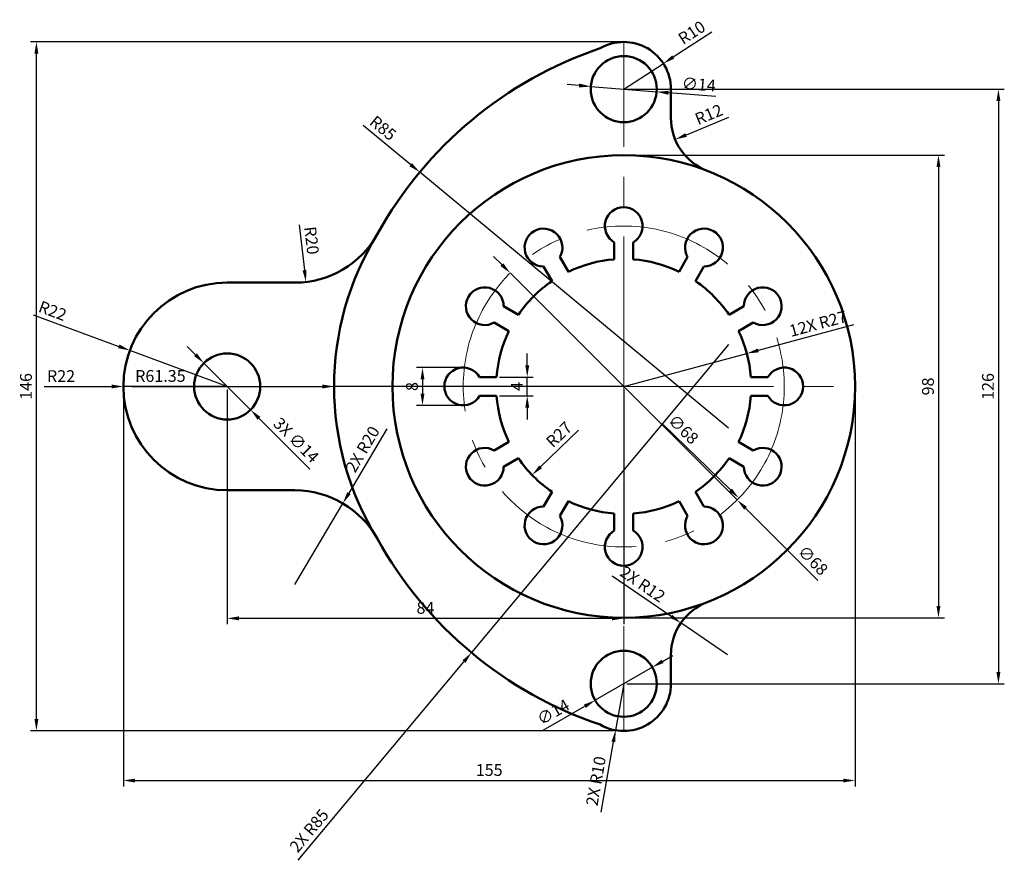
# Model space of a CAD drawing. Units: millimetres. Extents: x -56 to 153, y -43 to 135.
import ezdxf

# ---------------------------------------------------------------- set-up
doc = ezdxf.new("R2010")
doc.units = ezdxf.units.MM
doc.linetypes.add('CENTER', pattern=[50.8, 31.75, -6.35, 6.35, -6.35])
for name, color, linetype, lineweight in [('M-CNTR', 4, 'CENTER', 18), ('M-CONS', 8, 'Continuous', 13), ('M-DIMS', 2, 'Continuous', 25), ('M-OUTL', 7, 'Continuous', 50)]:
    doc.layers.add(name, color=color, linetype=linetype, lineweight=lineweight)
doc.styles.get("Standard").update_dxf_attribs({"font": 'arial.ttf'})
doc.dimstyles.new('ISO-25', dxfattribs={"dimtxt": 2.5, "dimasz": 2.5, "dimexe": 1.25, "dimexo": 0.625, "dimtad": 1, "dimtxsty": 'Standard', "dimcen": 2.5, "dimadec": 0, "dimazin": 0, "dimtfac": 1, "dimtmove": 0, "dimatfit": 3, "dimfxl": 1, "dimarcsym": 0})

# ---------------------------------------------------------------- blocks, each defined once
blk = doc.blocks.new('*U1')
for p, q in [((5.54, 2), (1.93, 2)), ((5.54, -2), (1.93, -2))]:
    blk.add_line(p, q)
blk.add_arc((-1.54, 0), 4, 30, 330)
blk = doc.blocks.new('*U2')
at = {"layer": 'M-OUTL', "color": 0, "linetype": 'ByBlock', "lineweight": -2, "transparency": 16777216}
for p, rotation in [((72.13, 89.86), 269.9999999999998), ((55.9, 85.51), 299.9999999999998), ((88.36, 85.51), 239.9999999999999), ((44.02, 73.63), 329.9999999999999), ((100.25, 73.63), 210), ((104.59, 57.4), 180), ((44.02, 41.16), 30), ((100.25, 41.16), 149.9999999999999), ((55.9, 29.28), 59.99999999999997), ((88.36, 29.28), 119.9999999999999), ((72.13, 24.93), 89.99999999999999)]:
    blk.add_blockref('*U1', p, dxfattribs=dict(at, rotation=rotation))
blk.add_blockref('*U1', (39.67, 57.4), dxfattribs=at)
blk = doc.blocks.new('*D3')
at = {"layer": 'Defpoints', "color": 0, "transparency": 16777216}
for p in [(94.13, 114.29), (83.03, 109.73)]:
    blk.add_point(p, dxfattribs=at)
at = {"layer": 'M-DIMS', "color": 0, "lineweight": -2, "transparency": 16777216}
blk.add_line((94.31, 114.37), (85.34, 110.68), dxfattribs=at)
at = {"layer": 'M-DIMS', "color": 0, "transparency": 16777216}
blk.add_solid([(85.18, 111.07), (85.5, 110.3), (83.03, 109.73)], dxfattribs=at)
at = {"layer": 'M-DIMS', "color": 0, "transparency": 16777216, "insert": (90.27, 114.74), "char_height": 2.5, "attachment_point": 5, "rotation": 22.3178}
blk.add_mtext('R12', dxfattribs=at)
blk = doc.blocks.new('*D4')
at = {"layer": 'Defpoints', "color": 0, "transparency": 16777216}
for p in [(65.15, 120.96), (79.11, 119.83)]:
    blk.add_point(p, dxfattribs=at)
at = {"layer": 'M-DIMS', "color": 0, "lineweight": -2, "transparency": 16777216}
for p, q in [((62.66, 121.16), (60.17, 121.37)), ((65.15, 120.96), (79.11, 119.83)), ((91.61, 118.81), (81.6, 119.63))]:
    blk.add_line(p, q, dxfattribs=at)
blk.add_arc((72.13, 120.4), 7, 345.1248, 354.8843, dxfattribs=at)
at = {"layer": 'M-DIMS', "color": 0, "transparency": 16777216}
for points in [[(62.7, 121.58), (62.63, 120.75), (65.15, 120.96)], [(81.63, 120.04), (81.57, 119.21), (79.11, 119.83)]]:
    blk.add_solid(points, dxfattribs=at)
at = {"layer": 'M-DIMS', "color": 0, "transparency": 16777216, "insert": (88.01, 121.08), "char_height": 2.5, "attachment_point": 5, "rotation": 355.3562}
blk.add_mtext('∅14', dxfattribs=at)
blk = doc.blocks.new('*D5')
at = {"layer": 'Defpoints', "color": 0, "transparency": 16777216}
for p in [(80.52, 125.84), (72.13, 120.4)]:
    blk.add_point(p, dxfattribs=at)
at = {"layer": 'M-DIMS', "color": 0, "lineweight": -2, "transparency": 16777216}
for p, q in [((90.77, 132.49), (82.62, 127.2)), ((72.13, 120.4), (80.52, 125.84))]:
    blk.add_line(p, q, dxfattribs=at)
at = {"layer": 'M-DIMS', "color": 0, "transparency": 16777216}
blk.add_solid([(82.39, 127.55), (82.84, 126.85), (80.52, 125.84)], dxfattribs=at)
at = {"layer": 'M-DIMS', "color": 0, "transparency": 16777216, "insert": (86.71, 132.12), "char_height": 2.5, "attachment_point": 5, "rotation": 32.9791}
blk.add_mtext('R10', dxfattribs=at)
blk = doc.blocks.new('*D6')
at = {"layer": 'Defpoints', "color": 0, "transparency": 16777216}
for p in [(72.13, 120.4), (72.13, -5.6), (151.5, -5.6)]:
    blk.add_point(p, dxfattribs=at)
at = {"layer": 'M-DIMS', "color": 0, "lineweight": -2, "transparency": 16777216}
for p, q in [((72.76, 120.4), (152.75, 120.4)), ((151.5, 117.9), (151.5, -3.1)), ((72.76, -5.6), (152.75, -5.6))]:
    blk.add_line(p, q, dxfattribs=at)
at = {"layer": 'M-DIMS', "color": 0, "transparency": 16777216}
for points in [[(151.08, 117.9), (151.92, 117.9), (151.5, 120.4)], [(151.08, -3.1), (151.92, -3.1), (151.5, -5.6)]]:
    blk.add_solid(points, dxfattribs=at)
at = {"layer": 'M-DIMS', "color": 0, "transparency": 16777216, "insert": (149.6, 57.4), "char_height": 2.5, "attachment_point": 5, "rotation": 90}
blk.add_mtext('126', dxfattribs=at)
blk = doc.blocks.new('*D7')
at = {"layer": 'Defpoints', "color": 0, "transparency": 16777216}
for p in [(72.13, 106.4), (72.13, 8.4), (138.8, 8.4)]:
    blk.add_point(p, dxfattribs=at)
at = {"layer": 'M-DIMS', "color": 0, "lineweight": -2, "transparency": 16777216}
for p, q in [((72.76, 106.4), (140.05, 106.4)), ((138.8, 103.9), (138.8, 10.9)), ((72.76, 8.4), (140.05, 8.4))]:
    blk.add_line(p, q, dxfattribs=at)
at = {"layer": 'M-DIMS', "color": 0, "transparency": 16777216}
for points in [[(138.38, 103.9), (139.22, 103.9), (138.8, 106.4)], [(138.38, 10.9), (139.22, 10.9), (138.8, 8.4)]]:
    blk.add_solid(points, dxfattribs=at)
at = {"layer": 'M-DIMS', "color": 0, "transparency": 16777216, "insert": (136.9, 57.4), "char_height": 2.5, "attachment_point": 5, "rotation": 90}
blk.add_mtext('98', dxfattribs=at)
blk = doc.blocks.new('*D8')
at = {"layer": 'Defpoints', "color": 0, "transparency": 16777216}
for p in [(72.13, 57.4), (52.72, 38.63)]:
    blk.add_point(p, dxfattribs=at)
at = {"layer": 'M-DIMS', "color": 0, "lineweight": -2, "transparency": 16777216}
blk.add_line((62.56, 48.14), (54.52, 40.37), dxfattribs=at)
at = {"layer": 'M-DIMS', "color": 0, "transparency": 16777216}
blk.add_solid([(54.23, 40.66), (54.81, 40.07), (52.72, 38.63)], dxfattribs=at)
at = {"layer": 'M-DIMS', "color": 0, "transparency": 16777216, "insert": (58.65, 46.98), "char_height": 2.5, "attachment_point": 5, "rotation": 44.0365}
blk.add_mtext('R27', dxfattribs=at)
blk = doc.blocks.new('*D9')
at = {"layer": 'Defpoints', "color": 0, "transparency": 16777216}
for p in [(47.72, 81.07), (96.54, 33.73)]:
    blk.add_point(p, dxfattribs=at)
at = {"layer": 'M-DIMS', "color": 0, "lineweight": -2, "transparency": 16777216}
blk.add_line((80.47, 49.31), (94.74, 35.47), dxfattribs=at)
at = {"layer": 'M-DIMS', "color": 0, "transparency": 16777216}
blk.add_solid([(95.03, 35.76), (94.45, 35.17), (96.54, 33.73)], dxfattribs=at)
at = {"layer": 'M-DIMS', "color": 0, "transparency": 16777216, "insert": (84.55, 48.09), "char_height": 2.5, "attachment_point": 5, "rotation": 315.8786}
blk.add_mtext('∅68', dxfattribs=at)
blk = doc.blocks.new('*D10')
at = {"layer": 'Defpoints', "color": 0, "transparency": 16777216}
for p in [(-32.5, 65.03), (-11.87, 57.4)]:
    blk.add_point(p, dxfattribs=at)
at = {"layer": 'M-DIMS', "color": 0, "lineweight": -2, "transparency": 16777216}
for p, q in [((-52.98, 72.6), (-34.85, 65.89)), ((-11.87, 57.4), (-32.5, 65.03))]:
    blk.add_line(p, q, dxfattribs=at)
at = {"layer": 'M-DIMS', "color": 0, "transparency": 16777216}
blk.add_solid([(-34.7, 66.29), (-34.99, 65.5), (-32.5, 65.03)], dxfattribs=at)
at = {"layer": 'M-DIMS', "color": 0, "transparency": 16777216, "insert": (-48.96, 73.12), "char_height": 2.5, "attachment_point": 5, "rotation": 339.7013}
blk.add_mtext('R22', dxfattribs=at)
blk = doc.blocks.new('*D11')
at = {"layer": 'Defpoints', "color": 0, "transparency": 16777216}
for p in [(2.49, 99.4), (4.81, 79.53)]:
    blk.add_point(p, dxfattribs=at)
at = {"layer": 'M-DIMS', "color": 0, "lineweight": -2, "transparency": 16777216}
blk.add_line((3.39, 91.66), (4.52, 82.01), dxfattribs=at)
at = {"layer": 'M-DIMS', "color": 0, "transparency": 16777216}
blk.add_solid([(4.93, 82.06), (4.1, 81.97), (4.81, 79.53)], dxfattribs=at)
at = {"layer": 'M-DIMS', "color": 0, "transparency": 16777216, "insert": (5.7, 88.3), "char_height": 2.5, "attachment_point": 5, "rotation": 276.6683}
blk.add_mtext('R20', dxfattribs=at)
blk = doc.blocks.new('*D12')
at = {"layer": 'Defpoints', "color": 0, "transparency": 16777216}
for p in [(-11.87, 57.4), (72.13, 57.4), (-11.87, 8.26)]:
    blk.add_point(p, dxfattribs=at)
at = {"layer": 'M-DIMS', "color": 0, "lineweight": -2, "transparency": 16777216}
for p, q in [((-11.87, 56.77), (-11.87, 7.01)), ((72.13, 56.77), (72.13, 7.01)), ((69.63, 8.26), (-9.37, 8.26))]:
    blk.add_line(p, q, dxfattribs=at)
at = {"layer": 'M-DIMS', "color": 0, "transparency": 16777216}
for points in [[(-9.37, 8.68), (-9.37, 7.84), (-11.87, 8.26)], [(69.63, 8.68), (69.63, 7.84), (72.13, 8.26)]]:
    blk.add_solid(points, dxfattribs=at)
at = {"layer": 'M-DIMS', "color": 0, "transparency": 16777216, "insert": (30.13, 10.16), "char_height": 2.5, "attachment_point": 5}
blk.add_mtext('84', dxfattribs=at)
blk = doc.blocks.new('*D13')
at = {"layer": 'Defpoints', "color": 0, "transparency": 16777216}
for p in [(38.37, 61.39), (29.5, 53.39), (38.37, 53.39)]:
    blk.add_point(p, dxfattribs=at)
at = {"layer": 'M-DIMS', "color": 0, "lineweight": -2, "transparency": 16777216}
for p, q in [((37.74, 61.39), (28.25, 61.39)), ((29.5, 58.89), (29.5, 55.89)), ((37.74, 53.39), (28.25, 53.39))]:
    blk.add_line(p, q, dxfattribs=at)
at = {"layer": 'M-DIMS', "color": 0, "transparency": 16777216}
for points in [[(29.09, 58.89), (29.92, 58.89), (29.5, 61.39)], [(29.09, 55.89), (29.92, 55.89), (29.5, 53.39)]]:
    blk.add_solid(points, dxfattribs=at)
at = {"layer": 'M-DIMS', "color": 0, "transparency": 16777216, "insert": (27.6, 57.39), "char_height": 2.5, "attachment_point": 5, "rotation": 90}
blk.add_mtext('8', dxfattribs=at)
blk = doc.blocks.new('*D14')
at = {"layer": 'Defpoints', "color": 0, "transparency": 16777216}
for p in [(45.21, 59.4), (51.69, 59.4), (45.21, 55.4)]:
    blk.add_point(p, dxfattribs=at)
at = {"layer": 'M-DIMS', "color": 0, "lineweight": -2, "transparency": 16777216}
for p, q in [((51.69, 61.9), (51.69, 64.4)), ((45.83, 59.4), (52.94, 59.4)), ((51.69, 55.4), (51.69, 59.4)), ((45.83, 55.4), (52.94, 55.4)), ((51.69, 52.9), (51.69, 50.4))]:
    blk.add_line(p, q, dxfattribs=at)
at = {"layer": 'M-DIMS', "color": 0, "transparency": 16777216}
for points in [[(51.28, 61.9), (52.11, 61.9), (51.69, 59.4)], [(51.28, 52.9), (52.11, 52.9), (51.69, 55.4)]]:
    blk.add_solid(points, dxfattribs=at)
at = {"layer": 'M-DIMS', "color": 0, "transparency": 16777216, "insert": (49.82, 57.4), "char_height": 2.5, "attachment_point": 5, "rotation": 90}
blk.add_mtext('4', dxfattribs=at)
blk = doc.blocks.new('*D15')
at = {"layer": 'Defpoints', "color": 0, "transparency": 16777216}
for p in [(28.92, 102.8), (94.34, 48.53)]:
    blk.add_point(p, dxfattribs=at)
at = {"layer": 'M-DIMS', "color": 0, "lineweight": -2, "transparency": 16777216}
for p, q in [((16.94, 112.75), (27, 104.4)), ((94.34, 48.53), (28.92, 102.8))]:
    blk.add_line(p, q, dxfattribs=at)
at = {"layer": 'M-DIMS', "color": 0, "transparency": 16777216}
blk.add_solid([(27.27, 104.72), (26.73, 104.08), (28.92, 102.8)], dxfattribs=at)
at = {"layer": 'M-DIMS', "color": 0, "transparency": 16777216, "insert": (20.94, 111.9), "char_height": 2.5, "attachment_point": 5, "rotation": 320.3196}
blk.add_mtext('R85', dxfattribs=at)
blk = doc.blocks.new('*D16')
at = {"layer": 'Defpoints', "color": 0, "transparency": 16777216}
for p in [(78.19, -2.1), (66.07, -9.11)]:
    blk.add_point(p, dxfattribs=at)
at = {"layer": 'M-DIMS', "color": 0, "lineweight": -2, "transparency": 16777216}
for p, q in [((80.36, -0.85), (82.52, 0.4)), ((78.19, -2.1), (66.07, -9.11)), ((55.07, -15.46), (63.91, -10.36))]:
    blk.add_line(p, q, dxfattribs=at)
at = {"layer": 'M-DIMS', "color": 0, "transparency": 16777216}
for points in [[(80.15, -0.49), (80.57, -1.21), (78.19, -2.1)], [(63.7, -10), (64.11, -10.72), (66.07, -9.11)]]:
    blk.add_solid(points, dxfattribs=at)
at = {"layer": 'M-DIMS', "color": 0, "transparency": 16777216, "insert": (57.35, -11.87), "char_height": 2.5, "attachment_point": 5, "rotation": 30.014}
blk.add_mtext('∅14', dxfattribs=at)
blk = doc.blocks.new('MOUNT-HOLE-D14')
blk.add_circle((7, 7), 7)
blk = doc.blocks.new('*D18')
at = {"layer": 'Defpoints', "color": 0, "transparency": 16777216}
for p in [(-52.28, 130.4), (72.13, 130.4), (72.13, -15.6)]:
    blk.add_point(p, dxfattribs=at)
at = {"layer": 'M-DIMS', "color": 0, "lineweight": -2, "transparency": 16777216}
for p, q in [((71.51, 130.4), (-53.53, 130.4)), ((-52.28, -13.1), (-52.28, 127.9)), ((71.51, -15.6), (-53.53, -15.6))]:
    blk.add_line(p, q, dxfattribs=at)
at = {"layer": 'M-DIMS', "color": 0, "transparency": 16777216}
for points in [[(-52.7, 127.9), (-51.87, 127.9), (-52.28, 130.4)], [(-52.7, -13.1), (-51.87, -13.1), (-52.28, -15.6)]]:
    blk.add_solid(points, dxfattribs=at)
at = {"layer": 'M-DIMS', "color": 0, "transparency": 16777216, "insert": (-54.18, 57.4), "char_height": 2.5, "attachment_point": 5, "rotation": 90}
blk.add_mtext('146', dxfattribs=at)
blk = doc.blocks.new('*D19')
at = {"layer": 'Defpoints', "color": 0, "transparency": 16777216}
for p in [(-33.87, 57.4), (121.13, 57.4), (121.13, -26.1)]:
    blk.add_point(p, dxfattribs=at)
at = {"layer": 'M-DIMS', "color": 0, "lineweight": -2, "transparency": 16777216}
for p, q in [((-33.87, 56.77), (-33.87, -27.35)), ((121.13, 56.77), (121.13, -27.35)), ((-31.37, -26.1), (118.63, -26.1))]:
    blk.add_line(p, q, dxfattribs=at)
at = {"layer": 'M-DIMS', "color": 0, "transparency": 16777216}
for points in [[(-31.37, -25.69), (-31.37, -26.52), (-33.87, -26.1)], [(118.63, -25.69), (118.63, -26.52), (121.13, -26.1)]]:
    blk.add_solid(points, dxfattribs=at)
at = {"layer": 'M-DIMS', "color": 0, "transparency": 16777216, "insert": (43.63, -24.2), "char_height": 2.5, "attachment_point": 5}
blk.add_mtext('155', dxfattribs=at)
blk = doc.blocks.new('*D20')
at = {"layer": 'Defpoints', "color": 0, "transparency": 16777216}
for p in [(94.34, 66.26), (39.88, 1)]:
    blk.add_point(p, dxfattribs=at)
at = {"layer": 'M-DIMS', "color": 0, "lineweight": -2, "transparency": 16777216}
for p, q in [((94.34, 66.26), (39.88, 1)), ((3.15, -43.01), (38.28, -0.92))]:
    blk.add_line(p, q, dxfattribs=at)
at = {"layer": 'M-DIMS', "color": 0, "transparency": 16777216}
blk.add_solid([(37.96, -0.65), (38.6, -1.18), (39.88, 1)], dxfattribs=at)
at = {"layer": 'M-DIMS', "color": 0, "transparency": 16777216, "insert": (5.74, -36.93), "char_height": 2.5, "attachment_point": 5, "rotation": 50.1525}
blk.add_mtext('2X R85', dxfattribs=at)
blk = doc.blocks.new('*D21')
at = {"layer": 'Defpoints', "color": 0, "transparency": 16777216}
for p in [(10.78, 57.39), (72.13, 57.4)]:
    blk.add_point(p, dxfattribs=at)
at = {"layer": 'M-DIMS', "color": 0, "lineweight": -2, "transparency": 16777216}
for p, q in [((-32.07, 57.39), (8.28, 57.39)), ((72.13, 57.4), (10.78, 57.39))]:
    blk.add_line(p, q, dxfattribs=at)
at = {"layer": 'M-DIMS', "color": 0, "transparency": 16777216}
blk.add_solid([(8.28, 57.81), (8.28, 56.98), (10.78, 57.39)], dxfattribs=at)
at = {"layer": 'M-DIMS', "color": 0, "transparency": 16777216, "insert": (-26.02, 59.3), "char_height": 2.5, "attachment_point": 5, "rotation": 0.0003}
blk.add_mtext('R61.35', dxfattribs=at)
blk = doc.blocks.new('*D22')
at = {"layer": 'Defpoints', "color": 0, "transparency": 16777216}
for p in [(48.09, 81.44), (96.17, 33.35)]:
    blk.add_point(p, dxfattribs=at)
at = {"layer": 'M-DIMS', "color": 0, "lineweight": -2, "transparency": 16777216}
for p, q in [((46.32, 83.21), (44.55, 84.97)), ((48.09, 81.44), (96.17, 33.35)), ((113.27, 16.26), (97.94, 31.59))]:
    blk.add_line(p, q, dxfattribs=at)
at = {"layer": 'M-DIMS', "color": 0, "transparency": 16777216}
for points in [[(46.62, 83.5), (46.03, 82.91), (48.09, 81.44)], [(98.24, 31.88), (97.65, 31.29), (96.17, 33.35)]]:
    blk.add_solid(points, dxfattribs=at)
at = {"layer": 'M-DIMS', "color": 0, "transparency": 16777216, "insert": (111.99, 20.32), "char_height": 2.5, "attachment_point": 5, "rotation": 314.9991}
blk.add_mtext('∅68', dxfattribs=at)
blk = doc.blocks.new('*D23')
at = {"layer": 'Defpoints', "color": 0, "transparency": 16777216}
for p in [(98.21, 64.38), (72.13, 57.4)]:
    blk.add_point(p, dxfattribs=at)
at = {"layer": 'M-DIMS', "color": 0, "lineweight": -2, "transparency": 16777216}
for p, q in [((120.77, 70.43), (100.63, 65.03)), ((72.13, 57.4), (98.21, 64.38))]:
    blk.add_line(p, q, dxfattribs=at)
at = {"layer": 'M-DIMS', "color": 0, "transparency": 16777216}
blk.add_solid([(100.52, 65.43), (100.73, 64.63), (98.21, 64.38)], dxfattribs=at)
at = {"layer": 'M-DIMS', "color": 0, "transparency": 16777216, "insert": (113.37, 70.39), "char_height": 2.5, "attachment_point": 5, "rotation": 14.9992}
blk.add_mtext('12X R27', dxfattribs=at)
blk = doc.blocks.new('*D24')
at = {"layer": 'Defpoints', "color": 0, "transparency": 16777216}
for p in [(-33.87, 57.39), (-11.87, 57.4)]:
    blk.add_point(p, dxfattribs=at)
at = {"layer": 'M-DIMS', "color": 0, "lineweight": -2, "transparency": 16777216}
for p, q in [((-50.67, 57.39), (-36.37, 57.39)), ((-11.87, 57.4), (-33.87, 57.39))]:
    blk.add_line(p, q, dxfattribs=at)
at = {"layer": 'M-DIMS', "color": 0, "transparency": 16777216}
blk.add_solid([(-36.37, 57.81), (-36.37, 56.98), (-33.87, 57.39)], dxfattribs=at)
at = {"layer": 'M-DIMS', "color": 0, "transparency": 16777216, "insert": (-47.07, 59.27), "char_height": 2.5, "attachment_point": 5, "rotation": 0.001}
blk.add_mtext('R22', dxfattribs=at)
blk = doc.blocks.new('*D25')
at = {"layer": 'Defpoints', "color": 0, "transparency": 16777216}
for p in [(12.64, 32.63), (2.49, 15.4)]:
    blk.add_point(p, dxfattribs=at)
at = {"layer": 'M-DIMS', "color": 0, "lineweight": -2, "transparency": 16777216}
for p, q in [((21.94, 48.4), (13.91, 34.78)), ((2.49, 15.4), (12.64, 32.63))]:
    blk.add_line(p, q, dxfattribs=at)
at = {"layer": 'M-DIMS', "color": 0, "transparency": 16777216}
blk.add_solid([(13.55, 34.99), (14.27, 34.57), (12.64, 32.63)], dxfattribs=at)
at = {"layer": 'M-DIMS', "color": 0, "transparency": 16777216, "insert": (17.09, 43.93), "char_height": 2.5, "attachment_point": 5, "rotation": 59.4893}
blk.add_mtext('2X R20', dxfattribs=at)
blk = doc.blocks.new('*D26')
at = {"layer": 'Defpoints', "color": 0, "transparency": 16777216}
for p in [(84.23, 7.29), (94.13, 0.5)]:
    blk.add_point(p, dxfattribs=at)
at = {"layer": 'M-DIMS', "color": 0, "lineweight": -2, "transparency": 16777216}
for p, q in [((69.71, 17.24), (82.17, 8.7)), ((94.13, 0.5), (84.23, 7.29))]:
    blk.add_line(p, q, dxfattribs=at)
at = {"layer": 'M-DIMS', "color": 0, "transparency": 16777216}
blk.add_solid([(82.41, 9.04), (81.94, 8.36), (84.23, 7.29)], dxfattribs=at)
at = {"layer": 'M-DIMS', "color": 0, "transparency": 16777216, "insert": (75.97, 15.23), "char_height": 2.5, "attachment_point": 5, "rotation": 325.5709}
blk.add_mtext('2X R12', dxfattribs=at)
blk = doc.blocks.new('*D27')
at = {"layer": 'Defpoints', "color": 0, "transparency": 16777216}
for p in [(72.13, -5.6), (70.4, -15.45)]:
    blk.add_point(p, dxfattribs=at)
at = {"layer": 'M-DIMS', "color": 0, "lineweight": -2, "transparency": 16777216}
for p, q in [((72.13, -5.6), (70.4, -15.45)), ((67.33, -32.81), (69.96, -17.91))]:
    blk.add_line(p, q, dxfattribs=at)
at = {"layer": 'M-DIMS', "color": 0, "transparency": 16777216}
blk.add_solid([(69.55, -17.84), (70.37, -17.99), (70.4, -15.45)], dxfattribs=at)
at = {"layer": 'M-DIMS', "color": 0, "transparency": 16777216, "insert": (66.56, -26.27), "char_height": 2.5, "attachment_point": 5, "rotation": 80.0009}
blk.add_mtext('2X R10', dxfattribs=at)
blk = doc.blocks.new('*D28')
at = {"layer": 'Defpoints', "color": 0, "transparency": 16777216}
for p in [(-16.82, 62.35), (-6.92, 52.45)]:
    blk.add_point(p, dxfattribs=at)
at = {"layer": 'M-DIMS', "color": 0, "lineweight": -2, "transparency": 16777216}
for p, q in [((-18.59, 64.11), (-20.35, 65.88)), ((-16.82, 62.35), (-6.92, 52.45)), ((5.65, 39.87), (-5.15, 50.68))]:
    blk.add_line(p, q, dxfattribs=at)
at = {"layer": 'M-DIMS', "color": 0, "transparency": 16777216}
for points in [[(-18.29, 64.41), (-18.88, 63.82), (-16.82, 62.35)], [(-4.86, 50.97), (-5.45, 50.38), (-6.92, 52.45)]]:
    blk.add_solid(points, dxfattribs=at)
at = {"layer": 'M-DIMS', "color": 0, "transparency": 16777216, "insert": (2.53, 45.79), "char_height": 2.5, "attachment_point": 5, "rotation": 314.9956}
blk.add_mtext('3X ∅14', dxfattribs=at)

msp = doc.modelspace()

# ---------------------------------------------------------------- linework, layer by layer
at = {"layer": 'M-CNTR'}
for p, q in [((72.131, 120.395), (72.131, 130.395)), ((72.131, 57.395), (72.131, 120.395)), ((10.784, 57.395), (-41.783, 57.395)), ((72.131, 57.395), (10.784, 57.395)), ((72.131, 57.395), (72.131, -5.605)), ((72.131, 57.395), (121.131, 57.395)), ((72.131, -5.605), (72.131, -15.605))]:
    msp.add_line(p, q, dxfattribs=at)
msp.add_circle((72.131, 57.395), 34, dxfattribs=at)
at = {"layer": 'M-CONS'}
for p, q in [((72.131, 120.395), (72.131, 120.395)), ((72.131, 120.395), (72.131, 120.395)), ((10.816, 59.395), (10.784, 59.395)), ((10.816, 55.395), (10.784, 55.395))]:
    msp.add_line(p, q, dxfattribs=at)
at = {"layer": 'M-OUTL'}
for p, q in [((82.131, 120.395), (82.131, 114.29)), ((-11.869, 79.395), (2.486, 79.395)), ((-11.869, 35.395), (2.486, 35.395)), ((82.131, -5.605), (82.131, 0.501))]:
    msp.add_line(p, q, dxfattribs=at)
msp.add_circle((72.131, 57.395), 49, dxfattribs=at)
for centre, radius, start, end in [((72.131, 120.395), 10, 0, 120), ((94.342, 48.529), 85, 108.6708, 151.02403), ((94.131, 114.29), 12, 180, 248.85953), ((2.486, 99.395), 20, 270, 331.02403), ((72.131, 57.395), 61.347, 148.21788, 211.78212), ((72.131, 57.395), 27, 94.24802, 115.75198), ((72.131, 57.395), 27, 64.24802, 85.75198), ((-11.869, 57.395), 22, 90, 270), ((72.131, 57.395), 27, 124.24802, 145.75198), ((72.131, 57.395), 27, 34.24802, 55.75198), ((72.131, 57.395), 27, 154.24802, 175.75198), ((72.131, 57.395), 27, 4.24802, 25.75198), ((72.131, 57.395), 27, 184.24802, 205.75198), ((72.131, 57.395), 27, 334.24802, 355.75198), ((72.131, 57.395), 27, 214.24802, 235.75198), ((72.131, 57.395), 27, 304.24802, 325.75198), ((2.486, 15.395), 20, 28.97597, 90), ((72.131, 57.395), 27, 244.24802, 265.75198), ((72.131, 57.395), 27, 274.24802, 295.75198), ((94.342, 66.262), 85, 208.97597, 251.3292), ((94.131, 0.501), 12, 111.14047, 180), ((72.131, -5.605), 10, 240, 0)]:
    msp.add_arc(centre, radius, start, end, dxfattribs=at)

# ---------------------------------------------------------------- block references
for name, p in [('MOUNT-HOLE-D14', (65.131, 113.395)), ('*U2', (0, 0)), ('MOUNT-HOLE-D14', (-18.869, 50.395)), ('MOUNT-HOLE-D14', (65.131, -12.605))]:
    msp.add_blockref(name, p, dxfattribs=at)

# ---------------------------------------------------------------- dimensions: what is measured, and where the dimension line sits
at = {"layer": 'M-DIMS'}
dim = msp.add_radius_dim(center=(72.131, 120.395), mpoint=(80.52, 125.839), dimstyle='ISO-25', override={"dimclrd": 0, "dimclre": 0, "dimclrt": 0}, dxfattribs=at)
dim.commit()
dim.dimension.update_dxf_attribs({"geometry": '*D5', "text_midpoint": (86.706, 132.119)})
for base, p1, p2, override, picture, middle in [((-52.283, 130.395), (72.131, -15.605), (72.131, 130.395), {"dimdec": 0, "dimlfac": 1, "dimrnd": 0, "dimzin": 0, "dimdsep": 46, "dimlunit": 2}, '*D18', (-54.185, 57.395)), ((151.5, -5.605), (72.131, 120.395), (72.131, -5.605), {"dimclrd": 0, "dimclre": 0, "dimclrt": 0}, '*D6', (149.598, 57.395)), ((138.799, 8.395), (72.131, 106.395), (72.131, 8.395), {"dimclrd": 0, "dimclre": 0, "dimclrt": 0}, '*D7', (136.898, 57.395)), ((51.692, 59.395), (45.206, 55.395), (45.206, 59.395), {"dimclrd": 0, "dimclre": 0, "dimclrt": 0}, '*D14', (49.817, 57.395)), ((29.504, 53.388), (38.367, 61.388), (38.367, 53.388), {"dimclrd": 0, "dimclre": 0, "dimclrt": 0}, '*D13', (27.603, 57.388))]:
    dim = msp.add_linear_dim(base=base, p1=p1, p2=p2, angle=90, dimstyle='ISO-25', override=override, dxfattribs=at)
    dim.commit()
    dim.dimension.update_dxf_attribs({"geometry": picture, "text_midpoint": middle})
dim = msp.add_diameter_dim_2p(p1=(65.154, 120.962), p2=(79.108, 119.829), dimstyle='ISO-25', override={"dimclrd": 0, "dimclre": 0, "dimclrt": 0}, dxfattribs=at)
dim.commit()
dim.dimension.update_dxf_attribs({"geometry": '*D4', "text_midpoint": (88.01, 121.083)})
for center, mpoint, override, picture, middle in [((94.131, 114.29), (83.03, 109.733), {"dimclrd": 0, "dimclre": 0, "dimclrt": 0}, '*D3', (90.985, 112.999)), ((94.342, 48.529), (28.925, 102.802), {"dimclrd": 0, "dimclre": 0, "dimclrt": 0}, '*D15', (19.724, 110.435)), ((2.486, 99.395), (4.808, 79.531), {"dimclrd": 0, "dimclre": 0, "dimclrt": 0}, '*D11', (3.809, 88.08)), ((-11.869, 57.395), (-32.502, 65.027), {"dimclrd": 0, "dimclre": 0, "dimclrt": 0}, '*D10', (-49.609, 71.355)), ((-11.869, 57.395), (-33.869, 57.395), {"dimdec": 0, "dimlfac": 1, "dimrnd": 0, "dimzin": 0, "dimdsep": 46, "dimlunit": 2}, '*D24', (-47.069, 57.395)), ((72.131, 57.395), (10.784, 57.395), {"dimdec": 2, "dimlfac": 1, "dimrnd": 0, "dimzin": 0, "dimdsep": 46, "dimlunit": 2}, '*D21', (-26.025, 57.395)), ((72.131, 57.395), (52.721, 38.627), {"dimclrd": 0, "dimclre": 0, "dimclrt": 0}, '*D8', (59.958, 45.625))]:
    dim = msp.add_radius_dim(center=center, mpoint=mpoint, dimstyle='ISO-25', override=override, dxfattribs=at)
    dim.commit()
    dim.dimension.update_dxf_attribs({"geometry": picture, "text_midpoint": middle, "dimtype": 164})
for p1, p2, override, picture, middle in [((48.09, 81.437), (96.173, 33.353), {"dimdec": 0, "dimlfac": 1, "dimrnd": 0, "dimzin": 0, "dimdsep": 46, "dimlunit": 2}, '*D22', (110.597, 18.928)), ((47.724, 81.066), (96.539, 33.725), {"dimclrd": 0, "dimclre": 0, "dimclrt": 0}, '*D9', (83.181, 46.68)), ((78.193, -2.103), (66.07, -9.106), {"dimclrd": 0, "dimclre": 0, "dimclrt": 0}, '*D16', (58.332, -13.576))]:
    dim = msp.add_diameter_dim_2p(p1=p1, p2=p2, dimstyle='ISO-25', override=override, dxfattribs=at)
    dim.commit()
    dim.dimension.update_dxf_attribs({"geometry": picture, "text_midpoint": middle, "dimtype": 163})
for center, mpoint, text, picture, middle in [((72.131, 57.395), (98.211, 64.383), '12X <>', '*D23', (113.86, 68.576)), ((94.342, 66.262), (39.879, 1.003), '2X <>', '*D20', (7.201, -38.152)), ((2.486, 15.395), (12.64, 32.626), '2X <>', '*D25', (18.732, 42.964))]:
    dim = msp.add_radius_dim(center=center, mpoint=mpoint, text=text, dimstyle='ISO-25', override={"dimdec": 0, "dimlfac": 1, "dimrnd": 0, "dimzin": 0, "dimdsep": 46, "dimlunit": 2}, dxfattribs=at)
    dim.commit()
    dim.dimension.update_dxf_attribs({"geometry": picture, "text_midpoint": middle, "dimtype": 164})
dim = msp.add_diameter_dim_2p(p1=(-16.818, 62.345), p2=(-6.919, 52.445), text='3X <>', dimstyle='ISO-25', override={"dimdec": 0, "dimlfac": 1, "dimrnd": 0, "dimzin": 0, "dimdsep": 46, "dimlunit": 2}, dxfattribs=at)
dim.commit()
dim.dimension.update_dxf_attribs({"geometry": '*D28', "text_midpoint": (1.133, 44.391), "dimtype": 163})
for base, p1, p2, override, picture, middle in [((121.131, -26.105), (-33.869, 57.395), (121.131, 57.395), {"dimdec": 0, "dimlfac": 1, "dimrnd": 0, "dimzin": 0, "dimdsep": 46, "dimlunit": 2}, '*D19', (43.631, -24.203)), ((-11.869, 8.259), (72.131, 57.395), (-11.869, 57.395), {"dimclrd": 0, "dimclre": 0, "dimclrt": 0}, '*D12', (30.131, 10.161))]:
    dim = msp.add_linear_dim(base=base, p1=p1, p2=p2, dimstyle='ISO-25', override=override, dxfattribs=at)
    dim.commit()
    dim.dimension.update_dxf_attribs({"geometry": picture, "text_midpoint": middle})
for center, mpoint, picture, middle in [((94.131, 0.501), (84.233, 7.285), '*D26', (75.971, 15.229)), ((72.131, -5.605), (70.395, -15.453), '*D27', (66.558, -26.266))]:
    dim = msp.add_radius_dim(center=center, mpoint=mpoint, text='2X <>', dimstyle='ISO-25', override={"dimdec": 0, "dimlfac": 1, "dimrnd": 0, "dimzin": 0, "dimdsep": 46, "dimlunit": 2}, dxfattribs=at)
    dim.commit()
    dim.dimension.update_dxf_attribs({"geometry": picture, "text_midpoint": middle})

doc.saveas('drawing.dxf')
